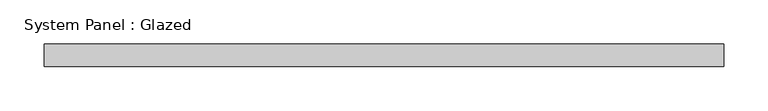
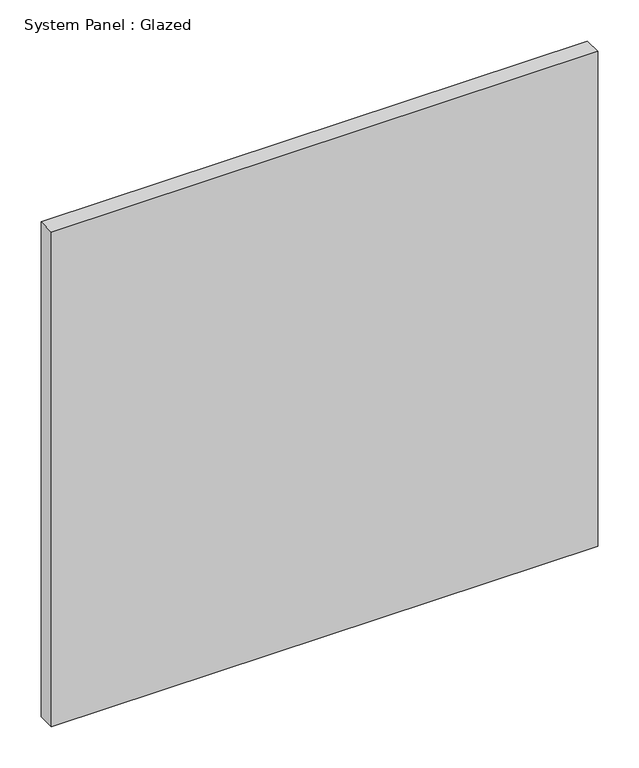
"""IFC4 building model written with IfcOpenShell, lengths in millimetres: plate geometry, System Panel : Glazed."""

from ifc_helpers import new_model, si_unit, origin, origin_with_axes, place, context, project, spatial, polyline, outline, extrude, source, transform, mapped, element, save


def system_panel_glazed_8f137235(model_context):
    return source(origin(), model_context, "Body", "SweptSolid", [
        extrude(outline(polyline([(384.175, 19.05), (-384.175, 19.05), (-384.175, 44.45), (384.175, 44.45), (384.175, 19.05)])), origin_with_axes(), (0.0, 0.0, 1.0), 735.4244987),
    ])


if __name__ == "__main__":
    model = new_model("IFC4")
    model_context = context("Model", 3, world=origin())
    ifc_project = project(units=[si_unit("LENGTHUNIT", "METRE", prefix="MILLI")], contexts=[model_context])
    site = spatial("IfcSite", under=ifc_project)
    building = spatial("IfcBuilding", under=site)
    placement = place(None, origin())
    system_panel_glazed_shape = system_panel_glazed_8f137235(model_context)
    element("IfcPlate", 1, ObjectType="System Panel : Glazed", at=placement, inside=building, context=model_context, shape_type="MappedRepresentation", body=[
        mapped(system_panel_glazed_shape, transform((0.0, 0.0, 0.0), x_axis=(1.0, 0.0, 0.0), y_axis=(0.0, 1.0, 0.0), z_axis=(0.0, 0.0, 1.0))),
    ])
    save(model, "model.ifc")

# Revit data of these elements
# Type "System Panel : Glazed"
#   Construction Type Id = "GSP4R"
#   Analytic Construction = "1/8 in Pilkington single glazing"
#   Visual Light Transmittance = 0.9
#   Solar Heat Gain Coefficient = 0.86
#   Heat Transfer Coefficient (U) = 1.18115 BTU/(h·ft²·°F)
#   Define Thermal Properties by = 1
# Element 1 (IfcPlate, "System Panel : Glazed")
#   Materials on its faces: "Glass"
# Materials
#   "Glass": class "Glass", colour RGB 0 128 192, transparency 0.75, Description = "Soda Lime Glass", Cost = 0
